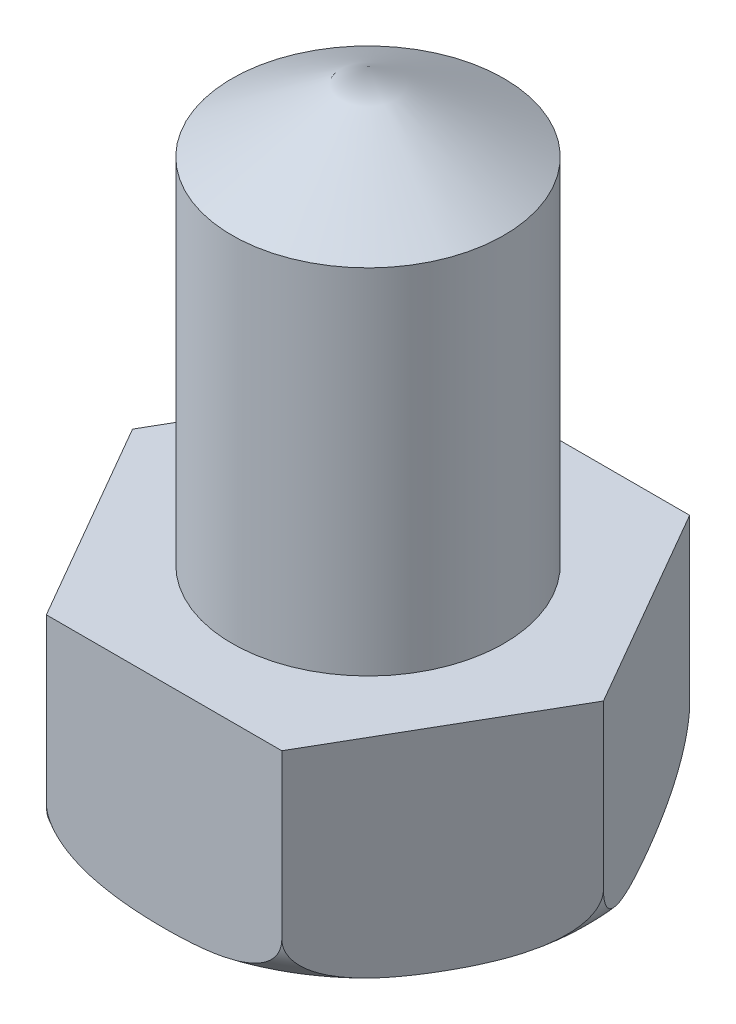
SolidWorks part; units mm, degrees
material "Plain Carbon Steel"
ref_plane "Front Plane" through (0, 0, 0) normal (0, 0, 1) x (1, 0, 0)
ref_plane "Top Plane" through (0, 0, 0) normal (0, 1, 0) x (1, 0, 0)
ref_plane "Right Plane" through (0, 0, 0) normal (1, 0, 0) x (0, 0, -1)
sketch "Hex Head Profile" plane through (0, 0, 0) normal (0, 1, 0) x (1, 0, 0)
  line L1 (8.6603, 0) -> (4.3301, 7.5)
  line L2 (4.3301, 7.5) -> (-4.3301, 7.5)
  line L3 (-4.3301, 7.5) -> (-8.6603, 0)
  line L4 (-8.6603, 0) -> (-4.3301, -7.5)
  line L5 (-4.3301, -7.5) -> (4.3301, -7.5)
  line L6 (4.3301, -7.5) -> (8.6603, 0)
  circle A0 centre (0, 0) radius 7.5 construction
  dimension "D1" = 15
extrude "Hex Head 15AF" add sketch "Hex Head Profile" along normal blind 8
sketch "Shank Profile" plane through (0, 0, 0) normal (0, 0, 1) x (1, 0, 0)
  line L0 (0, 8) -> (0, 23.8868)
  line L1 (0, 23.8868) -> (5, 21)
  line L2 (5, 21) -> (5, 8)
  line L3 (-4.3301, 8) -> (4.3301, 8) construction
  line L4 (0, 8) -> (5, 8)
  line L5 (0, 23.8868) -> (0, 35.3056) construction
  dimension "D1" = 120
  dimension "D2" = 5
  dimension "D3" = 13
revolve "Shank with Cone Point" add sketch "Shank Profile" angle 360 about L5
sketch "Head Chamfer Profile" plane through (0, 0, 0) normal (0, 0, 1) x (1, 0, 0)
  line L0 (0, 0) -> (0, 4.6316) construction
  line L1 (8.6603, 0) -> (6.6603, 0)
  line L2 (4.3301, 0) -> (8.6603, 0) construction
  line L3 (8.6603, 2) -> (8.6603, 0)
  line L4 (-4.3301, 0) -> (4.3301, 0) construction
  arc A0 (6.6603, 0) -> (8.6603, 2) centre (6.6603, 2) ccw
  dimension "D1" = 2
revolve "Head Chamfer Cut" cut sketch "Head Chamfer Profile" angle 360 about L0
